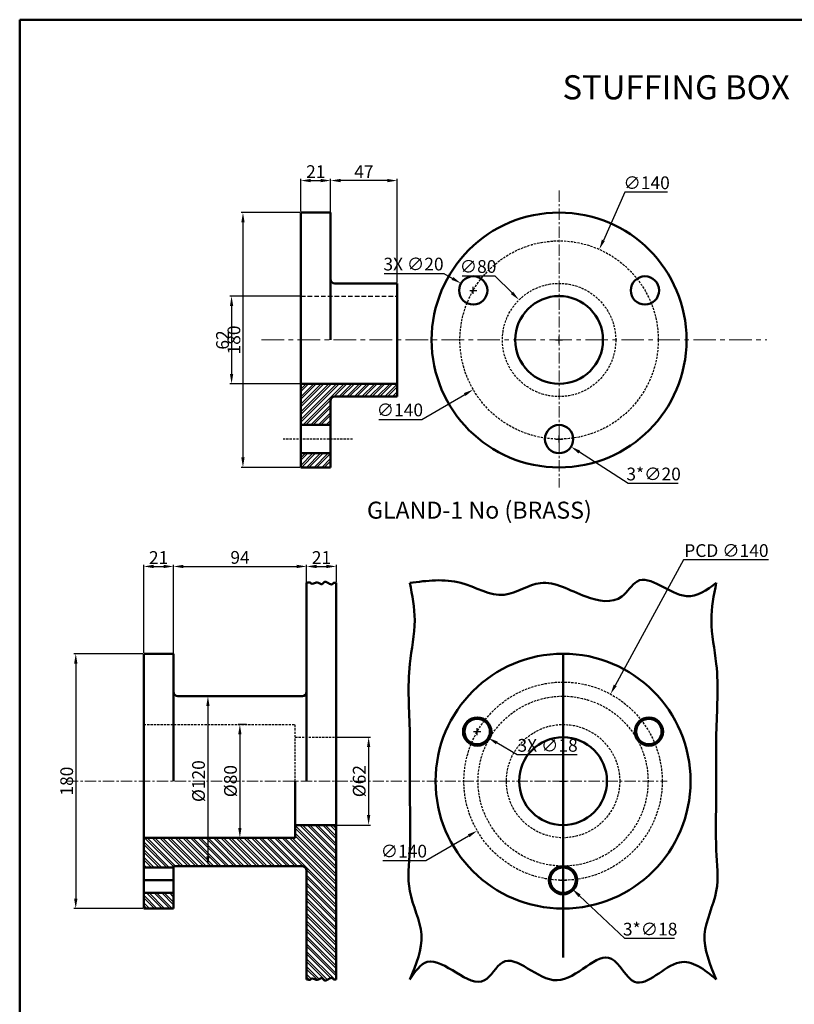
# Model space of a CAD drawing. Units: millimetres. Extents: x -98 to 907, y -783 to 313.
# Tile 2 of 3: x -98 to 449, y -383 to 313. Entities that reach past the tile are written whole.
import ezdxf

# ---------------------------------------------------------------- set-up
doc = ezdxf.new("R2010")
doc.units = ezdxf.units.MM
doc.header["$LTSCALE"] = 0.5
doc.linetypes.add('CENTER', pattern=[50.8, 31.75, -6.35, 6.35, -6.35])
doc.linetypes.add('HIDDEN', pattern=[9.525, 6.35, -3.175])
for name, color, linetype, lineweight in [('M-CNTR', 1, 'CENTER', 18), ('M-DIMS', 2, 'Continuous', 25), ('M-HATC', 8, 'Continuous', 18), ('M-HIDN', 4, 'HIDDEN', 25), ('M-OUTL', 7, 'Continuous', 50), ('M-TEXT', 3, 'Continuous', 25)]:
    doc.layers.add(name, color=color, linetype=linetype, lineweight=lineweight)
doc.styles.get("Standard").update_dxf_attribs({"font": 'arial.ttf'})
doc.dimstyles.new('ISO-25', dxfattribs={"dimtxt": 9, "dimasz": 7, "dimexe": 1.25, "dimexo": 0.625, "dimtad": 1, "dimtoh": 1, "dimtxsty": 'Standard', "dimcen": 2.5, "dimadec": 0, "dimazin": 0, "dimtfac": 1, "dimtofl": 0, "dimtmove": 0, "dimatfit": 3, "dimfxl": 1, "dimarcsym": 0})

# ---------------------------------------------------------------- blocks, each defined once
blk = doc.blocks.new('*D1')
at = {"layer": 'Defpoints', "color": 0, "ltscale": 0.5, "transparency": 16777216}
for p in [(100.46, 176.62), (59.55, -3.38), (100.46, -3.38)]:
    blk.add_point(p, dxfattribs=at)
at = {"layer": 'M-DIMS', "color": 0, "lineweight": -2, "ltscale": 0.5, "transparency": 16777216}
for p, q in [((99.83, 176.62), (58.3, 176.62)), ((59.55, 169.62), (59.55, 3.62)), ((99.83, -3.38), (58.3, -3.38))]:
    blk.add_line(p, q, dxfattribs=at)
at = {"layer": 'M-DIMS', "color": 0, "ltscale": 0.5, "transparency": 16777216}
for points in [[(58.38, 169.62), (60.72, 169.62), (59.55, 176.62)], [(58.38, 3.62), (60.72, 3.62), (59.55, -3.38)]]:
    blk.add_solid(points, dxfattribs=at)
at = {"layer": 'M-DIMS', "color": 0, "ltscale": 0.5, "transparency": 16777216, "insert": (54.33, 86.62), "char_height": 9, "attachment_point": 5, "rotation": 90}
blk.add_mtext('180', dxfattribs=at)
blk = doc.blocks.new('*D2')
at = {"layer": 'Defpoints', "color": 0, "ltscale": 0.5, "transparency": 16777216}
for p in [(121.46, 199.21), (100.46, 176.62), (121.46, 176.62)]:
    blk.add_point(p, dxfattribs=at)
at = {"layer": 'M-DIMS', "color": 0, "lineweight": -2, "ltscale": 0.5, "transparency": 16777216}
for p, q in [((100.46, 177.25), (100.46, 200.46)), ((107.46, 199.21), (114.46, 199.21)), ((121.46, 177.25), (121.46, 200.46))]:
    blk.add_line(p, q, dxfattribs=at)
at = {"layer": 'M-DIMS', "color": 0, "ltscale": 0.5, "transparency": 16777216}
for points in [[(107.46, 200.38), (107.46, 198.04), (100.46, 199.21)], [(114.46, 200.38), (114.46, 198.04), (121.46, 199.21)]]:
    blk.add_solid(points, dxfattribs=at)
at = {"layer": 'M-DIMS', "color": 0, "ltscale": 0.5, "transparency": 16777216, "insert": (110.96, 204.35), "char_height": 9, "attachment_point": 5}
blk.add_mtext('21', dxfattribs=at)
blk = doc.blocks.new('*D3')
at = {"layer": 'Defpoints', "color": 0, "ltscale": 0.5, "transparency": 16777216}
for p in [(121.46, 199.21), (168.46, 126.62), (121.46, 111.18)]:
    blk.add_point(p, dxfattribs=at)
at = {"layer": 'M-DIMS', "color": 0, "lineweight": -2, "ltscale": 0.5, "transparency": 16777216}
for p, q in [((121.46, 111.81), (121.46, 200.46)), ((161.46, 199.21), (128.46, 199.21)), ((168.46, 127.25), (168.46, 200.46))]:
    blk.add_line(p, q, dxfattribs=at)
at = {"layer": 'M-DIMS', "color": 0, "ltscale": 0.5, "transparency": 16777216}
for points in [[(128.46, 200.38), (128.46, 198.04), (121.46, 199.21)], [(161.46, 200.38), (161.46, 198.04), (168.46, 199.21)]]:
    blk.add_solid(points, dxfattribs=at)
at = {"layer": 'M-DIMS', "color": 0, "ltscale": 0.5, "transparency": 16777216, "insert": (144.96, 204.34), "char_height": 9, "attachment_point": 5}
blk.add_mtext('47', dxfattribs=at)
blk = doc.blocks.new('*D4')
at = {"layer": 'Defpoints', "color": 0, "ltscale": 0.5, "transparency": 16777216}
for p in [(311.19, 150.59), (254.36, 22.65)]:
    blk.add_point(p, dxfattribs=at)
at = {"layer": 'M-DIMS', "color": 0, "lineweight": -2, "ltscale": 0.5, "transparency": 16777216}
for p, q in [((329.13, 191), (314.03, 156.99)), ((359.4, 191), (329.13, 191)), ((280.27, 86.62), (285.27, 86.62)), ((282.77, 84.12), (282.77, 89.12))]:
    blk.add_line(p, q, dxfattribs=at)
at = {"layer": 'M-DIMS', "color": 0, "ltscale": 0.5, "transparency": 16777216}
blk.add_solid([(312.96, 157.47), (315.1, 156.52), (311.19, 150.59)], dxfattribs=at)
at = {"layer": 'M-DIMS', "color": 0, "ltscale": 0.5, "transparency": 16777216, "insert": (344.58, 196.47), "char_height": 9, "attachment_point": 5}
blk.add_mtext('∅140', dxfattribs=at)
blk = doc.blocks.new('*D5')
at = {"layer": 'Defpoints', "color": 0, "ltscale": 0.5, "transparency": 16777216}
for p in [(274.35, 22.01), (291.2, 11.23)]:
    blk.add_point(p, dxfattribs=at)
at = {"layer": 'M-DIMS', "color": 0, "lineweight": -2, "ltscale": 0.5, "transparency": 16777216}
for p, q in [((280.27, 16.62), (285.27, 16.62)), ((282.77, 14.12), (282.77, 19.12)), ((331.63, -14.67), (297.09, 7.45)), ((366.77, -14.67), (331.63, -14.67))]:
    blk.add_line(p, q, dxfattribs=at)
at = {"layer": 'M-DIMS', "color": 0, "ltscale": 0.5, "transparency": 16777216}
blk.add_solid([(297.72, 8.43), (296.46, 6.47), (291.2, 11.23)], dxfattribs=at)
at = {"layer": 'M-DIMS', "color": 0, "ltscale": 0.5, "transparency": 16777216, "insert": (349.51, -9.2), "char_height": 9, "attachment_point": 5}
blk.add_mtext('3*∅20', dxfattribs=at)
blk = doc.blocks.new('*D6')
at = {"layer": 'Defpoints', "color": 0, "ltscale": 0.5, "transparency": 16777216}
for p in [(-10.51, -134.96), (-58.5, -314.96), (-10.51, -314.96)]:
    blk.add_point(p, dxfattribs=at)
at = {"layer": 'M-DIMS', "color": 0, "lineweight": -2, "ltscale": 0.5, "transparency": 16777216}
for p, q in [((-11.14, -134.96), (-59.75, -134.96)), ((-58.5, -141.96), (-58.5, -307.96)), ((-11.14, -314.96), (-59.75, -314.96))]:
    blk.add_line(p, q, dxfattribs=at)
at = {"layer": 'M-DIMS', "color": 0, "ltscale": 0.5, "transparency": 16777216}
for points in [[(-59.67, -141.96), (-57.33, -141.96), (-58.5, -134.96)], [(-59.67, -307.96), (-57.33, -307.96), (-58.5, -314.96)]]:
    blk.add_solid(points, dxfattribs=at)
at = {"layer": 'M-DIMS', "color": 0, "ltscale": 0.5, "transparency": 16777216, "insert": (-63.72, -224.96), "char_height": 9, "attachment_point": 5, "rotation": 90}
blk.add_mtext('180', dxfattribs=at)
blk = doc.blocks.new('*D7')
at = {"layer": 'Defpoints', "color": 0, "ltscale": 0.5, "transparency": 16777216}
for p in [(42.98, -164.96), (34.81, -284.96), (42.98, -284.96)]:
    blk.add_point(p, dxfattribs=at)
at = {"layer": 'M-DIMS', "color": 0, "lineweight": -2, "ltscale": 0.5, "transparency": 16777216}
for p, q in [((42.36, -164.96), (33.56, -164.96)), ((34.81, -171.96), (34.81, -277.96)), ((42.36, -284.96), (33.56, -284.96))]:
    blk.add_line(p, q, dxfattribs=at)
at = {"layer": 'M-DIMS', "color": 0, "ltscale": 0.5, "transparency": 16777216}
for points in [[(33.64, -171.96), (35.97, -171.96), (34.81, -164.96)], [(33.64, -277.96), (35.97, -277.96), (34.81, -284.96)]]:
    blk.add_solid(points, dxfattribs=at)
at = {"layer": 'M-DIMS', "color": 0, "ltscale": 0.5, "transparency": 16777216, "insert": (29.34, -224.96), "char_height": 9, "attachment_point": 5, "rotation": 90}
blk.add_mtext('%%C120', dxfattribs=at)
blk = doc.blocks.new('*D8')
at = {"layer": 'Defpoints', "color": 0, "ltscale": 0.5, "transparency": 16777216}
for p in [(62.61, -184.96), (57.37, -264.96), (62.61, -264.96)]:
    blk.add_point(p, dxfattribs=at)
at = {"layer": 'M-DIMS', "color": 0, "lineweight": -2, "ltscale": 0.5, "transparency": 16777216}
for p, q in [((61.98, -184.96), (56.12, -184.96)), ((57.37, -191.96), (57.37, -257.96)), ((61.98, -264.96), (56.12, -264.96))]:
    blk.add_line(p, q, dxfattribs=at)
at = {"layer": 'M-DIMS', "color": 0, "ltscale": 0.5, "transparency": 16777216}
for points in [[(56.21, -191.96), (58.54, -191.96), (57.37, -184.96)], [(56.21, -257.96), (58.54, -257.96), (57.37, -264.96)]]:
    blk.add_solid(points, dxfattribs=at)
at = {"layer": 'M-DIMS', "color": 0, "ltscale": 0.5, "transparency": 16777216, "insert": (51.9, -224.96), "char_height": 9, "attachment_point": 5, "rotation": 90}
blk.add_mtext('%%C80', dxfattribs=at)
blk = doc.blocks.new('*D9')
at = {"layer": 'Defpoints', "color": 0, "ltscale": 0.5, "transparency": 16777216}
for p in [(125.49, -193.96), (125.49, -255.96), (148.29, -255.96)]:
    blk.add_point(p, dxfattribs=at)
at = {"layer": 'M-DIMS', "color": 0, "lineweight": -2, "ltscale": 0.5, "transparency": 16777216}
for p, q in [((126.11, -193.96), (149.54, -193.96)), ((148.29, -200.96), (148.29, -248.96)), ((126.11, -255.96), (149.54, -255.96))]:
    blk.add_line(p, q, dxfattribs=at)
at = {"layer": 'M-DIMS', "color": 0, "ltscale": 0.5, "transparency": 16777216}
for points in [[(147.12, -200.96), (149.46, -200.96), (148.29, -193.96)], [(147.12, -248.96), (149.46, -248.96), (148.29, -255.96)]]:
    blk.add_solid(points, dxfattribs=at)
at = {"layer": 'M-DIMS', "color": 0, "ltscale": 0.5, "transparency": 16777216, "insert": (142.82, -224.96), "char_height": 9, "attachment_point": 5, "rotation": 90}
blk.add_mtext('%%C62', dxfattribs=at)
blk = doc.blocks.new('*D10')
at = {"layer": 'Defpoints', "color": 0, "ltscale": 0.5, "transparency": 16777216}
for p in [(10.49, -73.34), (-10.51, -134.96), (10.49, -134.96)]:
    blk.add_point(p, dxfattribs=at)
at = {"layer": 'M-DIMS', "color": 0, "lineweight": -2, "ltscale": 0.5, "transparency": 16777216}
for p, q in [((-10.51, -134.34), (-10.51, -72.09)), ((-3.51, -73.34), (3.49, -73.34)), ((10.49, -134.34), (10.49, -72.09))]:
    blk.add_line(p, q, dxfattribs=at)
at = {"layer": 'M-DIMS', "color": 0, "ltscale": 0.5, "transparency": 16777216}
for points in [[(-3.51, -72.17), (-3.51, -74.51), (-10.51, -73.34)], [(3.49, -72.17), (3.49, -74.51), (10.49, -73.34)]]:
    blk.add_solid(points, dxfattribs=at)
at = {"layer": 'M-DIMS', "color": 0, "ltscale": 0.5, "transparency": 16777216, "insert": (-0.01, -68.2), "char_height": 9, "attachment_point": 5}
blk.add_mtext('21', dxfattribs=at)
blk = doc.blocks.new('*D11')
at = {"layer": 'Defpoints', "color": 0, "ltscale": 0.5, "transparency": 16777216}
for p in [(104.49, -73.34), (10.49, -144.94), (104.49, -144.94)]:
    blk.add_point(p, dxfattribs=at)
at = {"layer": 'M-DIMS', "color": 0, "lineweight": -2, "ltscale": 0.5, "transparency": 16777216}
for p, q in [((10.49, -144.31), (10.49, -72.09)), ((17.49, -73.34), (97.49, -73.34)), ((104.49, -144.31), (104.49, -72.09))]:
    blk.add_line(p, q, dxfattribs=at)
at = {"layer": 'M-DIMS', "color": 0, "ltscale": 0.5, "transparency": 16777216}
for points in [[(17.49, -72.17), (17.49, -74.51), (10.49, -73.34)], [(97.49, -72.17), (97.49, -74.51), (104.49, -73.34)]]:
    blk.add_solid(points, dxfattribs=at)
at = {"layer": 'M-DIMS', "color": 0, "ltscale": 0.5, "transparency": 16777216, "insert": (57.49, -68.12), "char_height": 9, "attachment_point": 5}
blk.add_mtext('94', dxfattribs=at)
blk = doc.blocks.new('*D12')
at = {"layer": 'Defpoints', "color": 0, "ltscale": 0.5, "transparency": 16777216}
for p in [(125.49, -73.34), (104.49, -84.96), (125.49, -84.96)]:
    blk.add_point(p, dxfattribs=at)
at = {"layer": 'M-DIMS', "color": 0, "lineweight": -2, "ltscale": 0.5, "transparency": 16777216}
for p, q in [((104.49, -84.34), (104.49, -72.09)), ((111.49, -73.34), (118.49, -73.34)), ((125.49, -84.34), (125.49, -72.09))]:
    blk.add_line(p, q, dxfattribs=at)
at = {"layer": 'M-DIMS', "color": 0, "ltscale": 0.5, "transparency": 16777216}
for points in [[(111.49, -72.17), (111.49, -74.51), (104.49, -73.34)], [(118.49, -72.17), (118.49, -74.51), (125.49, -73.34)]]:
    blk.add_solid(points, dxfattribs=at)
at = {"layer": 'M-DIMS', "color": 0, "ltscale": 0.5, "transparency": 16777216, "insert": (114.99, -68.2), "char_height": 9, "attachment_point": 5}
blk.add_mtext('21', dxfattribs=at)
blk = doc.blocks.new('*D13')
at = {"layer": 'Defpoints', "color": 0, "ltscale": 0.5, "transparency": 16777216}
for p in [(279.03, -288.79), (292.12, -301.14)]:
    blk.add_point(p, dxfattribs=at)
at = {"layer": 'M-DIMS', "color": 0, "lineweight": -2, "ltscale": 0.5, "transparency": 16777216}
for p, q in [((283.07, -294.96), (288.07, -294.96)), ((285.57, -297.46), (285.57, -292.46)), ((329.18, -336.12), (297.21, -305.95)), ((364.37, -336.12), (329.18, -336.12))]:
    blk.add_line(p, q, dxfattribs=at)
at = {"layer": 'M-DIMS', "color": 0, "ltscale": 0.5, "transparency": 16777216}
blk.add_solid([(298.01, -305.1), (296.41, -306.8), (292.12, -301.14)], dxfattribs=at)
at = {"layer": 'M-DIMS', "color": 0, "ltscale": 0.5, "transparency": 16777216, "insert": (347.08, -330.65), "char_height": 9, "attachment_point": 5}
blk.add_mtext('3*∅18', dxfattribs=at)
blk = doc.blocks.new('*D14')
at = {"layer": 'Defpoints', "color": 0, "ltscale": 0.5, "transparency": 16777216}
for p in [(319.07, -163.5), (252.08, -286.43)]:
    blk.add_point(p, dxfattribs=at)
at = {"layer": 'M-DIMS', "color": 0, "lineweight": -2, "ltscale": 0.5, "transparency": 16777216}
for p, q in [((370.69, -68.76), (322.42, -157.35)), ((430.54, -68.76), (370.69, -68.76)), ((285.57, -227.46), (285.57, -222.46)), ((283.07, -224.96), (288.07, -224.96))]:
    blk.add_line(p, q, dxfattribs=at)
at = {"layer": 'M-DIMS', "color": 0, "ltscale": 0.5, "transparency": 16777216}
blk.add_solid([(321.39, -156.79), (323.44, -157.91), (319.07, -163.5)], dxfattribs=at)
at = {"layer": 'M-DIMS', "color": 0, "ltscale": 0.5, "transparency": 16777216, "insert": (400.92, -63.29), "char_height": 9, "attachment_point": 5}
blk.add_mtext('PCD ∅140', dxfattribs=at)
blk = doc.blocks.new('*D37')
at = {"layer": 'Defpoints', "color": 0, "ltscale": 0.5, "transparency": 16777216}
for p in [(100.46, 117.62), (51.51, 55.62), (100.46, 55.62)]:
    blk.add_point(p, dxfattribs=at)
at = {"layer": 'M-DIMS', "color": 0, "lineweight": -2, "ltscale": 0.5, "transparency": 16777216}
for p, q in [((99.83, 117.62), (50.26, 117.62)), ((51.51, 110.62), (51.51, 62.62)), ((99.83, 55.62), (50.26, 55.62))]:
    blk.add_line(p, q, dxfattribs=at)
at = {"layer": 'M-DIMS', "color": 0, "ltscale": 0.5, "transparency": 16777216}
for points in [[(50.35, 110.62), (52.68, 110.62), (51.51, 117.62)], [(50.35, 62.62), (52.68, 62.62), (51.51, 55.62)]]:
    blk.add_solid(points, dxfattribs=at)
at = {"layer": 'M-DIMS', "color": 0, "ltscale": 0.5, "transparency": 16777216, "insert": (46.29, 86.62), "char_height": 9, "attachment_point": 5, "rotation": 90}
blk.add_mtext('62', dxfattribs=at)
blk = doc.blocks.new('*D47')
at = {"layer": 'Defpoints', "color": 0, "ltscale": 0.5, "transparency": 16777216}
for p in [(254.49, 114.91), (311.06, 58.33)]:
    blk.add_point(p, dxfattribs=at)
at = {"layer": 'M-DIMS', "color": 0, "lineweight": -2, "ltscale": 0.5, "transparency": 16777216}
for p, q in [((214.25, 131.88), (237.52, 131.88)), ((237.52, 131.88), (249.54, 119.86)), ((280.27, 86.62), (285.27, 86.62)), ((282.77, 84.12), (282.77, 89.12))]:
    blk.add_line(p, q, dxfattribs=at)
at = {"layer": 'M-DIMS', "color": 0, "ltscale": 0.5, "transparency": 16777216}
blk.add_solid([(250.37, 120.68), (248.72, 119.03), (254.49, 114.91)], dxfattribs=at)
at = {"layer": 'M-DIMS', "color": 0, "ltscale": 0.5, "transparency": 16777216, "insert": (225.57, 137.35), "char_height": 9, "attachment_point": 5}
blk.add_mtext('∅80', dxfattribs=at)
blk = doc.blocks.new('*D48')
at = {"layer": 'Defpoints', "color": 0, "ltscale": 0.5, "transparency": 16777216}
for p in [(343.38, 121.66), (222.17, 51.58)]:
    blk.add_point(p, dxfattribs=at)
at = {"layer": 'M-DIMS', "color": 0, "lineweight": -2, "ltscale": 0.5, "transparency": 16777216}
for p, q in [((280.27, 86.62), (285.27, 86.62)), ((282.77, 84.12), (282.77, 89.12)), ((185.81, 30.56), (216.11, 48.08)), ((155.54, 30.56), (185.81, 30.56))]:
    blk.add_line(p, q, dxfattribs=at)
at = {"layer": 'M-DIMS', "color": 0, "ltscale": 0.5, "transparency": 16777216}
blk.add_solid([(215.53, 49.09), (216.7, 47.07), (222.17, 51.58)], dxfattribs=at)
at = {"layer": 'M-DIMS', "color": 0, "ltscale": 0.5, "transparency": 16777216, "insert": (170.36, 36.04), "char_height": 9, "attachment_point": 5}
blk.add_mtext('∅140', dxfattribs=at)
blk = doc.blocks.new('*D49')
at = {"layer": 'Defpoints', "color": 0, "ltscale": 0.5, "transparency": 16777216}
for p in [(213.49, 126.61), (230.82, 116.63)]:
    blk.add_point(p, dxfattribs=at)
at = {"layer": 'M-DIMS', "color": 0, "lineweight": -2, "ltscale": 0.5, "transparency": 16777216}
for p, q in [((159.22, 133.59), (201.35, 133.59)), ((201.35, 133.59), (207.42, 130.1)), ((219.65, 121.62), (224.65, 121.62)), ((222.15, 119.12), (222.15, 124.12))]:
    blk.add_line(p, q, dxfattribs=at)
at = {"layer": 'M-DIMS', "color": 0, "ltscale": 0.5, "transparency": 16777216}
blk.add_solid([(208, 131.11), (206.84, 129.09), (213.49, 126.61)], dxfattribs=at)
at = {"layer": 'M-DIMS', "color": 0, "ltscale": 0.5, "transparency": 16777216, "insert": (179.97, 139.06), "char_height": 9, "attachment_point": 5}
blk.add_mtext('3X ∅20', dxfattribs=at)
blk = doc.blocks.new('*D50')
at = {"layer": 'Defpoints', "color": 0, "ltscale": 0.5, "transparency": 16777216}
for p in [(346.17, -189.91), (224.98, -260.01)]:
    blk.add_point(p, dxfattribs=at)
at = {"layer": 'M-DIMS', "color": 0, "lineweight": -2, "ltscale": 0.5, "transparency": 16777216}
for p, q in [((285.57, -227.46), (285.57, -222.46)), ((283.07, -224.96), (288.07, -224.96)), ((188.62, -281.04), (218.92, -263.52)), ((158.35, -281.04), (188.62, -281.04))]:
    blk.add_line(p, q, dxfattribs=at)
at = {"layer": 'M-DIMS', "color": 0, "ltscale": 0.5, "transparency": 16777216}
blk.add_solid([(218.33, -262.51), (219.5, -264.53), (224.98, -260.01)], dxfattribs=at)
at = {"layer": 'M-DIMS', "color": 0, "ltscale": 0.5, "transparency": 16777216, "insert": (173.17, -275.57), "char_height": 9, "attachment_point": 5}
blk.add_mtext('∅140', dxfattribs=at)
blk = doc.blocks.new('*D51')
at = {"layer": 'Defpoints', "color": 0, "ltscale": 0.5, "transparency": 16777216}
for p in [(217.16, -185.46), (232.74, -194.47)]:
    blk.add_point(p, dxfattribs=at)
at = {"layer": 'M-DIMS', "color": 0, "lineweight": -2, "ltscale": 0.5, "transparency": 16777216}
for p, q in [((224.95, -192.46), (224.95, -187.46)), ((222.45, -189.96), (227.45, -189.96)), ((253.26, -206.32), (238.8, -197.97)), ((295.44, -206.32), (253.26, -206.32))]:
    blk.add_line(p, q, dxfattribs=at)
at = {"layer": 'M-DIMS', "color": 0, "ltscale": 0.5, "transparency": 16777216}
blk.add_solid([(239.39, -196.96), (238.22, -198.98), (232.74, -194.47)], dxfattribs=at)
at = {"layer": 'M-DIMS', "color": 0, "ltscale": 0.5, "transparency": 16777216, "insert": (274.66, -200.85), "char_height": 9, "attachment_point": 5}
blk.add_mtext('3X ∅18', dxfattribs=at)

msp = doc.modelspace()

# ---------------------------------------------------------------- hatches: boundary and pattern name
at = {"layer": 'M-HATC', "ltscale": 0.5}
h = msp.add_hatch(dxfattribs=at)
h.set_pattern_fill('ANSI32', color=256, scale=0.4)
h.paths.add_polyline_path([(121.455, 6.6202), (100.455, 6.6202), (100.455, -3.3798), (121.455, -3.3798)])
h.paths.add_polyline_path([(121.455, 43.6202, -0.41421356), (124.455, 46.6202), (168.455, 46.6202), (168.455, 55.6202), (100.455, 55.6202), (100.455, 26.6202), (121.455, 26.6202)])
h = msp.add_hatch(dxfattribs=at)
h.set_pattern_fill('ANSI32', color=256, scale=0.4, angle=90)
h.set_pattern_definition([(135, (-144.1703, 20.2153), (-2.694077, -2.694077), []), (135, (-144.1703, 22.0113), (-2.694077, -2.694077), [])])
edge = h.paths.add_edge_path()
edge.add_line((-10.5144, -264.9638), (-10.5144, -285.9638))
edge.add_line((-10.5144, -285.9638), (10.4856, -285.9638))
edge.add_arc((11.4856, -285.9638), 1, 90, 180, ccw=False)
edge.add_line((11.4856, -284.9638), (101.4856, -284.9638))
edge.add_arc((101.4856, -287.9638), 3, 0, 90, ccw=False)
edge.add_line((104.4856, -287.9638), (104.4856, -364.9638))
edge.add_spline(control_points=[(104.4856, -364.9638), (105.5479, -365.2706), (106.8361, -365.6426), (107.9135, -364.159), (109.8798, -364.5013), (112.1661, -366.3126), (115.3201, -362.7805), (117.5301, -367.929), (121.5866, -362.4805), (123.475, -365.233), (124.6382, -365.0772), (125.4856, -364.9638)], knot_values=[0, 0, 0, 0, 2.79565042, 3.38979218, 5.12535939, 7.79423565, 11.48125794, 13.70150623, 19.51408934, 20.36796662, 22.65887887, 22.65887887, 22.65887887, 22.65887887], degree=3, periodic=0)
edge.add_line((125.4856, -364.9638), (125.4856, -255.9638))
edge.add_line((125.4856, -255.9638), (96.4856, -255.9638))
edge.add_line((96.4856, -255.9638), (96.4856, -264.9638))
edge.add_line((96.4856, -264.9638), (-10.5144, -264.9638))
h.paths.add_polyline_path([(-10.5144, -303.9638), (-10.5144, -314.9638), (10.4856, -314.9638), (10.4856, -303.9638)], flags=17)

# ---------------------------------------------------------------- linework, layer by layer
at = {"layer": 'M-CNTR', "ltscale": 0.5}
for p, q in [((282.7749, 192.159), (282.7749, -17.6738)), ((-64.713, -224.9638), (359.0597, -224.9638))]:
    msp.add_line(p, q, dxfattribs=at)
at = {"layer": 'M-CNTR'}
msp.add_line((72.7643, 86.6202), (429.4703, 86.6202), dxfattribs=at)
at = {"layer": 'M-HIDN'}
msp.add_line((100.455, 117.6202), (168.455, 117.6202), dxfattribs=at)
at = {"layer": 'M-HIDN', "ltscale": 0.5}
for p, q in [((136.9839, 16.6202), (88.0041, 16.6202)), ((-10.5144, -184.9638), (96.4856, -184.9638)), ((96.4856, -224.9638), (96.4856, -184.9638)), ((96.4856, -193.9638), (125.4856, -193.9638))]:
    msp.add_line(p, q, dxfattribs=at)
for centre, radius in [((282.7749, 86.6202), 70), ((282.7749, 86.6202), 40), ((285.5718, -224.9638), 70), ((285.5718, -224.9638), 60), ((285.5718, -224.9638), 40)]:
    msp.add_circle(centre, radius, dxfattribs=at)
at = {"layer": 'M-OUTL'}
for p, q in [((100.455, 176.6202), (100.455, -3.3798)), ((121.455, 176.6202), (100.455, 176.6202)), ((121.455, 86.6202), (121.455, 176.6202)), ((168.455, 126.6202), (124.455, 126.6202)), ((168.455, 46.6202), (168.455, 126.6202)), ((100.455, 55.6202), (168.455, 55.6202)), ((121.455, -3.3798), (121.455, 43.6202)), ((168.455, 46.6202), (124.455, 46.6202)), ((100.455, -3.3798), (121.455, -3.3798))]:
    msp.add_line(p, q, dxfattribs=at)
at = {"layer": 'M-OUTL', "ltscale": 0.5}
for p, q in [((121.455, 26.6202), (100.455, 26.6202)), ((121.455, 6.6202), (100.455, 6.6202)), ((104.4856, -161.9638), (104.4856, -84.9638)), ((125.4856, -84.9638), (125.4856, -364.9638)), ((-10.5144, -134.9638), (-10.5144, -314.9638)), ((10.4856, -134.9638), (-10.5144, -134.9638)), ((10.4856, -224.9638), (10.4856, -134.9638)), ((285.5718, -134.9638), (285.5718, -349.6004)), ((13.4856, -164.9638), (101.4856, -164.9638)), ((104.4856, -224.9638), (104.4856, -161.9638)), ((96.4856, -264.9638), (96.4856, -224.9638)), ((96.4856, -255.9638), (125.4856, -255.9638)), ((-10.5144, -264.9638), (96.4856, -264.9638)), ((11.4856, -284.9638), (101.4856, -284.9638)), ((-10.5144, -285.9638), (10.4856, -285.9638)), ((10.4856, -314.9638), (10.4856, -285.9638)), ((104.4856, -364.9638), (104.4856, -287.9638)), ((-10.5144, -294.9638), (10.4856, -294.9638)), ((-10.5144, -303.9638), (10.4856, -303.9638)), ((-10.5144, -314.9638), (10.4856, -314.9638))]:
    msp.add_line(p, q, dxfattribs=at)
msp.add_lwpolyline([(-98.0885, 312.8308), (906.5931, 312.8308), (906.5931, -783.1771), (-98.0885, -783.1771)], close=True, dxfattribs=at)
for centre, radius in [((282.7749, 86.6202), 90), ((222.1532, 121.6202), 10), ((343.3967, 121.6202), 10), ((282.7749, 86.6202), 31), ((282.7749, 16.6202), 10), ((285.5718, -224.9638), 90), ((224.95, -189.9638), 10), ((346.1936, -189.9638), 10), ((224.95, -189.9638), 9), ((346.1936, -189.9638), 9), ((285.5718, -224.9638), 31), ((285.5718, -294.9638), 10), ((285.5718, -294.9638), 9)]:
    msp.add_circle(centre, radius, dxfattribs=at)
at = {"layer": 'M-OUTL'}
for centre, start, end in [((124.455, 129.6202), 180, 270), ((124.455, 43.6202), 90, 180)]:
    msp.add_arc(centre, 3, start, end, dxfattribs=at)
at = {"layer": 'M-OUTL', "ltscale": 0.5}
for centre, radius, start, end in [((13.4856, -161.9638), 3, 180, 270), ((101.4856, -161.9638), 3, 270, 0), ((11.4856, -285.9638), 1, 90, 180), ((101.4856, -287.9638), 3, 0, 90)]:
    msp.add_arc(centre, radius, start, end, dxfattribs=at)
for points, knots in [([(104.4856, -84.9638), (105.5479, -84.657), (106.8361, -84.285), (107.9135, -85.7685), (109.8798, -85.4262), (112.1661, -83.615), (115.3201, -87.1471), (117.5301, -81.9986), (121.5866, -87.4471), (123.475, -84.6945), (124.6382, -84.8503), (125.4856, -84.9638)], [0, 0, 0, 0, 2.79565042, 3.38979218, 5.12535939, 7.79423565, 11.48125794, 13.70150623, 19.51408934, 20.36796662, 22.65887887, 22.65887887, 22.65887887, 22.65887887]), ([(177.3695, -84.9638), (189.4866, -83.3699), (212.317, -80.367), (242.4534, -99.8467), (271.9618, -78.307), (297.5522, -95.3997), (326.1645, -100.8476), (341.0384, -72.6862), (369.5354, -102.6319), (386.9964, -89.9042), (393.7741, -84.9638)], [0, 0, 0, 0, 36.00870346, 67.84594523, 94.59517974, 128.04743365, 153.49152427, 168.67480028, 205.05951054, 228.14243766, 228.14243766, 228.14243766, 228.14243766]), ([(177.3695, -84.9638), (179.1094, -93.7696), (182.871, -112.8076), (174.7284, -148.1703), (178.2358, -189.6961), (176.8232, -233.6003), (178.4984, -270.5538), (174.2351, -303.928), (190.6816, -333.5494), (181.844, -354.4048), (177.3695, -364.9638)], [0, 0, 0, 0, 26.6513058, 57.61925096, 106.86657481, 150.94275014, 189.28294753, 218.10715148, 249.93193945, 282.56837361, 282.56837361, 282.56837361, 282.56837361]), ([(393.7741, -84.9638), (392.0342, -93.7696), (388.2726, -112.8076), (396.4151, -148.1703), (392.9078, -189.6961), (394.3204, -233.6003), (392.6452, -270.5538), (396.9085, -303.928), (380.462, -333.5494), (389.2996, -354.4048), (393.7741, -364.9638)], [0, 0, 0, 0, 26.6513058, 57.61925096, 106.86657481, 150.94275014, 189.28294753, 218.10715148, 249.93193945, 282.56837361, 282.56837361, 282.56837361, 282.56837361]), ([(177.3695, -364.9638), (181.1468, -359.4311), (194.1185, -340.4308), (226.4306, -380.929), (246.403, -338.6838), (282.0398, -385.2215), (317.178, -333.7808), (337.0383, -380.5119), (366.5978, -342.7623), (385.2857, -358.0293), (393.7741, -364.9638)], [0, 0, 0, 0, 17.45434219, 59.94152025, 77.82300409, 118.32225016, 159.71255517, 182.80593211, 217.27191764, 245.95509139, 245.95509139, 245.95509139, 245.95509139]), ([(104.4856, -364.9638), (105.5479, -365.2706), (106.8361, -365.6426), (107.9135, -364.159), (109.8798, -364.5013), (112.1661, -366.3126), (115.3201, -362.7805), (117.5301, -367.929), (121.5866, -362.4805), (123.475, -365.233), (124.6382, -365.0772), (125.4856, -364.9638)], [0, 0, 0, 0, 2.79565042, 3.38979218, 5.12535939, 7.79423565, 11.48125794, 13.70150623, 19.51408934, 20.36796662, 22.65887887, 22.65887887, 22.65887887, 22.65887887])]:
    msp.add_open_spline(points, degree=3, knots=knots, dxfattribs=at)

# ---------------------------------------------------------------- texts
at = {"layer": 'M-TEXT', "ltscale": 0.5, "attachment_point": 1}
for s, insert, char_height in [('\\pxqc;STUFFING BOX', (274.8545, 273.5961), 17), ('\\pxqc;GLAND-1 No (BRASS)', (135.9088, -27.5769), 12)]:
    msp.add_mtext_dynamic_manual_height_columns(s, width=181.185119, gutter_width=12.5, heights=[0], dxfattribs=dict(at, insert=insert, char_height=char_height))

# ---------------------------------------------------------------- dimensions: what is measured, and where the dimension line sits
at = {"layer": 'M-DIMS', "ltscale": 0.5}
for base, p1, p2, picture, middle in [((121.455, 199.2108), (100.455, 176.6202), (121.455, 176.6202), '*D2', (110.955, 204.3542)), ((121.455, 199.2108), (168.455, 126.6202), (121.455, 111.1809), '*D3', (144.955, 204.3358)), ((10.4856, -73.34), (-10.5144, -134.9638), (10.4856, -134.9638), '*D10', (-0.0144, -68.1965)), ((104.4856, -73.34), (10.4856, -144.9367), (104.4856, -144.9367), '*D11', (57.4856, -68.1198)), ((125.4856, -73.34), (104.4856, -84.9638), (125.4856, -84.9638), '*D12', (114.9856, -68.1965))]:
    dim = msp.add_linear_dim(base=base, p1=p1, p2=p2, dimstyle='ISO-25', override={"dimclrd": 0, "dimclre": 0, "dimclrt": 0}, dxfattribs=at)
    dim.commit()
    dim.dimension.update_dxf_attribs({"geometry": picture, "text_midpoint": middle})
for p1, p2, override, picture, middle in [((254.3615, 22.6462), (311.1884, 150.5942), {"dimclrd": 0, "dimclre": 0, "dimclrt": 0}, '*D4', (344.5808, 190.9968)), ((311.0568, 58.3335), (254.4931, 114.9069), {"dimdec": 0, "dimlfac": 1, "dimrnd": 0, "dimzin": 0, "dimdsep": 46, "dimlunit": 2}, '*D47', (225.5723, 131.8789)), ((343.3762, 121.6557), (222.1736, 51.5848), {"dimdec": 0, "dimlfac": 1, "dimrnd": 0, "dimzin": 0, "dimdsep": 46, "dimlunit": 2}, '*D48', (170.3649, 30.5635)), ((346.1653, -189.9149), (224.9782, -260.0126), {"dimdec": 0, "dimlfac": 1, "dimrnd": 0, "dimzin": 0, "dimdsep": 46, "dimlunit": 2}, '*D50', (173.1741, -281.0419))]:
    dim = msp.add_diameter_dim_2p(p1=p1, p2=p2, dimstyle='ISO-25', override=override, dxfattribs=at)
    dim.commit()
    dim.dimension.update_dxf_attribs({"geometry": picture, "text_midpoint": middle, "dimtype": 163})
for base, p1, p2, override, picture, middle in [((59.5506, -3.3798), (100.455, 176.6202), (100.455, -3.3798), {"dimclrd": 0, "dimclre": 0, "dimclrt": 0}, '*D1', (54.3304, 86.6202)), ((51.5143, 55.6202), (100.455, 117.6202), (100.455, 55.6202), {"dimdec": 0, "dimlfac": 1, "dimrnd": 0, "dimzin": 0, "dimdsep": 46, "dimlunit": 2}, '*D37', (46.2942, 86.6202)), ((-58.5013, -314.9638), (-10.5144, -134.9638), (-10.5144, -314.9638), {"dimclrd": 0, "dimclre": 0, "dimclrt": 0}, '*D6', (-63.7215, -224.9638))]:
    dim = msp.add_linear_dim(base=base, p1=p1, p2=p2, angle=90, dimstyle='ISO-25', override=override, dxfattribs=at)
    dim.commit()
    dim.dimension.update_dxf_attribs({"geometry": picture, "text_midpoint": middle})
for p1, p2, text, override, picture, middle in [((230.8204, 116.6323), (213.4859, 126.6081), '3X <>', {"dimdec": 0, "dimlfac": 1, "dimrnd": 0, "dimzin": 0, "dimdsep": 46, "dimlunit": 2}, '*D49', (179.9734, 133.5911)), ((274.354, 22.0135), (291.1959, 11.2269), '3*<>', {"dimclrd": 0, "dimclre": 0, "dimclrt": 0}, '*D5', (349.5128, -14.6677)), ((252.0777, -286.4304), (319.0659, -163.4972), 'PCD <>', {"dimclrd": 0, "dimclre": 0, "dimclrt": 0}, '*D14', (400.9247, -68.7641)), ((279.027, -288.7859), (292.1166, -301.1416), '3*<>', {"dimclrd": 0, "dimclre": 0, "dimclrt": 0}, '*D13', (347.0848, -336.1225))]:
    dim = msp.add_diameter_dim_2p(p1=p1, p2=p2, text=text, dimstyle='ISO-25', override=override, dxfattribs=at)
    dim.commit()
    dim.dimension.update_dxf_attribs({"geometry": picture, "text_midpoint": middle, "dimtype": 163})
for base, p1, p2, picture, middle in [((34.8079, -284.9638), (42.9839, -164.9638), (42.9839, -284.9638), '*D7', (29.3361, -224.9638)), ((57.3736, -264.9638), (62.6062, -184.9638), (62.6062, -264.9638), '*D8', (51.9017, -224.9638)), ((148.2903, -255.9638), (125.4856, -193.9638), (125.4856, -255.9638), '*D9', (142.8184, -224.9638))]:
    dim = msp.add_linear_dim(base=base, p1=p1, p2=p2, angle=90, text='%%C<>', dimstyle='ISO-25', override={"dimclrd": 0, "dimclre": 0, "dimclrt": 0}, dxfattribs=at)
    dim.commit()
    dim.dimension.update_dxf_attribs({"geometry": picture, "text_midpoint": middle})
dim = msp.add_diameter_dim_2p(p1=(217.1575, -185.4608), p2=(232.7425, -194.4668), text='3X <>', dimstyle='ISO-25', override={"dimdec": 0, "dimlfac": 1, "dimrnd": 0, "dimzin": 0, "dimdsep": 46, "dimlunit": 2}, dxfattribs=at)
dim.commit()
dim.dimension.update_dxf_attribs({"geometry": '*D51', "text_midpoint": (274.6603, -206.3216)})

doc.saveas('drawing.dxf')
